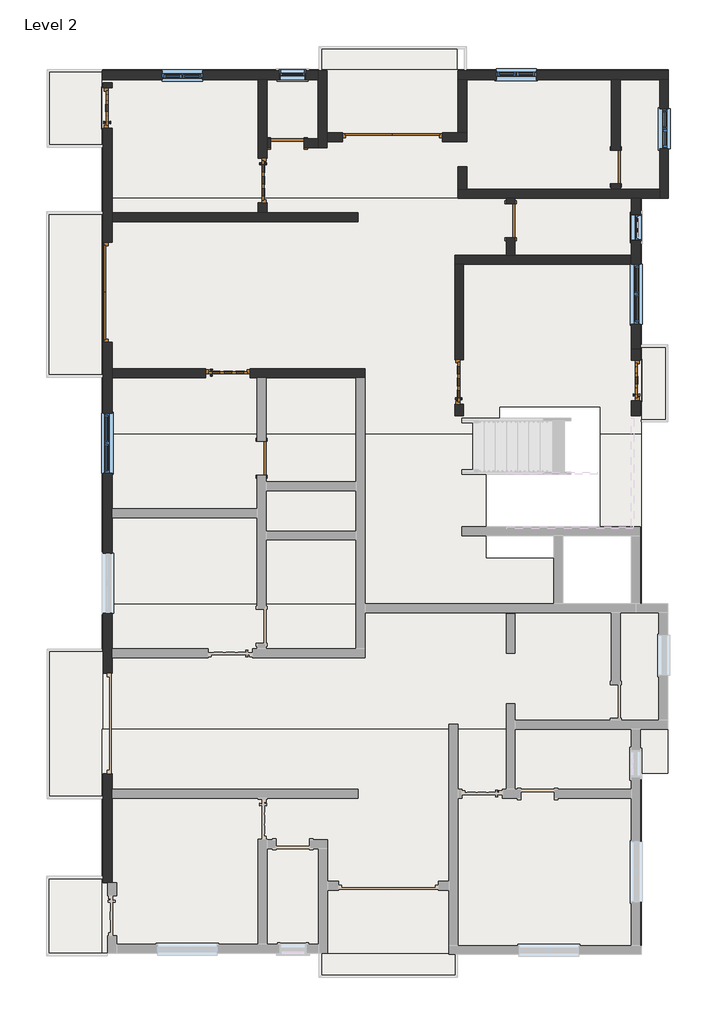
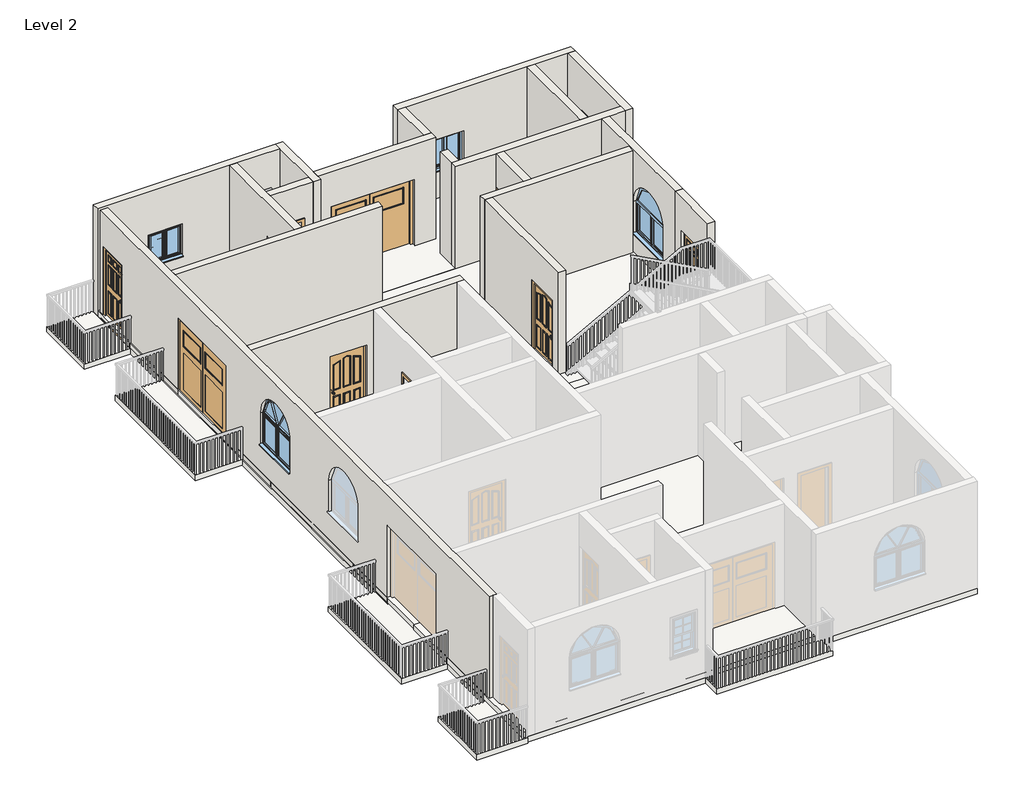
# One storey, part 2 of 7: 19 walls, 11 doors, 10 slabs, 7 windows, 5 roofs.
# Revit data of these elements (continued)
# Type "Windows_Dbl_w-Glazing_Bars : 910x910mm" (continued)
#   Type Mark = "33"
#   Operation = "DoublePanelVertical"
#   Construction Type Id = "GSP4R"
#   Manufacturer = "Revit"
#   Keynote = "L10"
#   Analytic Construction = "1/8 in Pilkington single glazing"
#   Wrap Layers (Ext) from Ext = 0' - 4.03543"
#   Wrap Layers (Int) from Ext = 0' - 6.98819"
#   Window Board Projection = 0' - 0.98425"
#   Window Board Extension = 0' - 0.98425"
#   Visual Light Transmittance = 0.9
#   Solar Heat Gain Coefficient = 0.78
#   Rough Width = 2' - 11.82677"
#   Rough Height = 2' - 11.82677"
#   Height = 2' - 11.82677"
#   Width = 2' - 11.82677"
#   Heat Transfer Coefficient (U) = 0.6496 BTU/(h·ft²·°F)
#   Glazing Thickness = 0' - 0.94488"
#   Glazing Bar Thickness = 0' - 0.7874"
#   FrameOffset - External = 0' - 1.9685"
#   Frame Depth = 0' - 2.55906"
#   Default Head Height = 6' - 10.67717"
#   Cill Depth = 0' - 3.44488"
#   Cavity Closer Width = 0' - 1.9685"
#   Cavity Closer Offset from Ext = 0' - 4.03543"
#   Cavity Closer Depth = 0' - 3.34646"
#   Vis - Glazing Bars = yes
#   Vis - Cavity Closers = yes
#   Define Thermal Properties by = 1
#   Material Trim = Window Frame
#   Material Glazing Bars = Window Frame
#   Material Glass = Glass
#   Material Frame = Window Frame
#   Wall Closure = (empty or 0)
# Elements 1, 2 (IfcDoor, "Doors_ExtSgl_5 : 910x2110mm")
#   Phase Created = New Construction
#   Materials on its faces: "Door - Panel", "Door - Handle", "Door - Frame/Mullion", "Door - Glazing"
# Elements 3, 4, 5 (IfcDoor, "Doors_ExtSgl_6 : 1010x2110mm")
#   Phase Created = New Construction
#   Materials on its faces: "Door - Panel", "Door - Handle", "Door - Frame/Mullion", "Door - Glazing"
# Element 6 (IfcDoor, "Doors_Garage_Timber_Side_Hung_Glazing : 2270x2050mm")
#   Phase Created = New Construction
#   Materials on its faces: "Door - Panel", "Door - Frame/Mullion", "Door - Glazing"
# Element 7 (IfcDoor, "Doors_Garage_Timber_Side_Hung_Glazing : 2270x2200mm")
#   Phase Created = New Construction
#   Materials on its faces: "Door - Panel", "Door - Frame/Mullion", "Door - Glazing"
# Elements 8, 9, 10, 11 (IfcDoor, "Single-Flush : 30\" x 80\"")
#   Phase Created = New Construction
#   Materials on its faces: "Door - Frame", "Door - Panel"
# Elements 12, 16 (IfcRoof, "Generic - 12\"")
#   built-in parameter 1001705 = 10.5 (stored number, unit not read)
#   built-in parameter 1001710 = 33615
#   Phase Created = New Construction
#   Materials on its faces: "Default Roof", "Earth"
# Element 13 (IfcRoof, "Generic - 12\"")
#   built-in parameter 1001705 = 10.5 (stored number, unit not read)
#   built-in parameter 1001710 = 33615
#   Phase Created = New Construction
#   Materials on its faces: "Default Roof"
# Element 14 (IfcRoof, "Generic - 12\"")
#   built-in parameter 1001705 = 10.5 (stored number, unit not read)
#   built-in parameter 1001710 = 33615
#   Phase Created = New Construction
#   Materials on its faces: "Default Roof", "Concrete, Lightweight"
# Element 15 (IfcRoof, "Generic - 12\"")
#   built-in parameter 1001705 = 10.5 (stored number, unit not read)
#   built-in parameter 1001710 = 33615
#   Phase Created = New Construction
#   Materials on its faces: "Default Roof", "Wood - Stained"
# Element 17 (IfcSlab, "Generic - 12\"")
#   Height Offset From Level = 0' - 0"
#   Phase Created = New Construction
#   Materials on its faces: "Default Floor", "Oak Flooring", "Concrete, Lightweight"
# Element 18 (IfcSlab, "Generic - 12\"")
#   Height Offset From Level = 0' - 0"
#   Phase Created = New Construction
#   Materials on its faces: "Default Floor", "Wood - Stained", "Concrete, Lightweight"
# Element 19 (IfcSlab, "Generic - 12\"")
#   Height Offset From Level = 0' - 0"
#   Phase Created = New Construction
#   Materials on its faces: "Default Floor", "Earth"
# Element 20 (IfcSlab, "Generic - 12\"")
#   Height Offset From Level = 0' - 0"
#   Phase Created = New Construction
#   Materials on its faces: "Default Floor", "mm"
# Elements 21, 22, 23, 24, 25 (IfcSlab, "Generic - 12\"")
#   Height Offset From Level = 0' - 0"
#   Phase Created = New Construction
#   Materials on its faces: "Default Floor"
# Element 26 (IfcSlab, "Generic - 12\"")
#   Height Offset From Level = 0' - 0"
#   Phase Created = New Construction
#   Materials on its faces: "Concrete, Lightweight", "Earth", "Default Floor"
# Elements 27, 31 (IfcWall, "Generic - 9\" w")
#   Top Offset = 0' - 0"
#   Base Offset = 0' - 0"
#   wall height = 10' - 0"
#   Phase Created = New Construction
#   Base Constraint = Level 2
#   Top Constraint = Level 3
#   Materials on its faces: "Default Wall", "Earth"
# Element 28 (IfcWall, "Generic - 9\" w")
#   Top Offset = 0' - 0"
#   Base Offset = 0' - 0"
#   wall height = 10' - 0"
#   Phase Created = New Construction
#   Base Constraint = Level 2
#   Top Constraint = Level 3
#   Materials on its faces: "Default Wall", "Wood - Stained"
# Element 29 (IfcWall, "Generic - 9\" w")
#   Top Offset = 0' - 0"
#   Base Offset = 0' - 0"
#   wall height = 10' - 0"
#   Phase Created = New Construction
#   Base Constraint = Level 2
#   Top Constraint = Level 3
#   Materials on its faces: "Default Wall", "Grass"
# Element 30 (IfcWall, "Generic - 9\" w")
#   Top Offset = 0' - 0"
#   Base Offset = 0' - 0"
#   wall height = 10' - 0"
#   Phase Created = New Construction
#   Base Constraint = Level 2
#   Top Constraint = Level 3
#   Materials on its faces: "Default Wall", "mm"
# Elements 32, 33, 35, 37, 38, 40, 41, 42, 43, 44, 45 (IfcWall, "Generic -4.5\" p")
#   Top Offset = 0' - 0"
#   Base Offset = 0' - 0"
#   wall height = 10' - 0"
#   Phase Created = New Construction
#   Base Constraint = Level 2
#   Top Constraint = Level 3
#   Materials on its faces: "Default Wall"
# Elements 34, 39 (IfcWall, "Generic -4.5\" p")
#   Top Offset = 0' - 0"
#   Base Offset = 0' - 0"
#   wall height = 10' - 0"
#   Phase Created = New Construction
#   Base Constraint = Level 2
#   Top Constraint = Level 3
#   Materials on its faces: "Default Wall", "Earth"
# Element 36 (IfcWall, "Generic -4.5\" p")
#   Top Offset = 0' - 0"
#   Base Offset = 0' - 0"
#   wall height = 10' - 0"
#   Phase Created = New Construction
#   Base Constraint = Level 2
#   Top Constraint = Level 3
#   Materials on its faces: "Default Wall", "Oak Flooring"
# Element 46 (IfcWindow, "Window-Double-Hung : 24\" x 42\"")
#   Mark = "24"
#   Window Inset = 0' - 0"
#   Interior Wall Closure = 0' - 1 1/2"
#   Frame Extension = 0' - 1 1/4"
#   Exterior Wall Closure = 0' - 0 1/2"
#   Interior Trim Visibility = yes
#   Indicator Visibility = yes
#   Exterior Trim Visibility = yes
#   Phase Created = New Construction
#   Materials on its faces: "Wood - Stained", "Glass", "Clad - White"
# Element 47 (IfcWindow, "Window-Double-Hung : 24\" x 42\"")
#   Mark = "30"
#   Window Inset = 0' - 0"
#   Interior Wall Closure = 0' - 1 1/2"
#   Frame Extension = 0' - 1 1/4"
#   Exterior Wall Closure = 0' - 0 1/2"
#   Interior Trim Visibility = yes
#   Indicator Visibility = yes
#   Exterior Trim Visibility = yes
#   Phase Created = New Construction
#   Materials on its faces: "Wood - Stained", "Glass", "Clad - White"
# Element 48 (IfcWindow, "Windows_Arched : 1360x910mm")
#   Mark = "20"
#   Phase Created = New Construction
#   Materials on its faces: "Window Frame", "Glass"
# Element 49 (IfcWindow, "Windows_Arched : 1360x910mm")
#   Mark = "31"
#   Phase Created = New Construction
#   Materials on its faces: "Window Frame", "Glass"
# Element 50 (IfcWindow, "Windows_Dbl_w-Glazing_Bars : 910x910mm")
#   Mark = "27"
#   Phase Created = New Construction
#   Materials on its faces: "Window Frame", "Glass"
# Element 51 (IfcWindow, "Windows_Dbl_w-Glazing_Bars : 910x910mm")
#   Mark = "28"
#   Phase Created = New Construction
#   Materials on its faces: "Window Frame", "Glass"
# Element 52 (IfcWindow, "Windows_Dbl_w-Glazing_Bars : 910x910mm")
#   Mark = "29"
#   Phase Created = New Construction
#   Materials on its faces: "Window Frame", "Glass"
# Materials
#   "Door - Glazing": colour RGB 0 0 255, transparency 0.75
#   "Door - Panel": class "Wood", colour RGB 210 159 95, transparency 0, Cost = 0
#   "Door - Frame/Mullion": class "Wood", colour RGB 212 179 113, transparency 0
#   "Door - Handle": colour RGB 0 0 0, transparency 0
#   "Door - Frame": colour RGB 118 70 51, transparency 0, Cost = 0
#   "Wood - Stained": class "Wood", colour RGB 224 178 126, transparency 0, Cost = 0
#   "Clad - White": class "Wood", colour RGB 242 242 238, transparency 0, Cost = 0
#   "Glass": class "Glass", colour RGB 0 128 192, transparency 0.75, Description = "Soda Lime Glass", Cost = 0
#   "Window Frame": colour RGB 249 249 249, transparency 0
#   "Default Roof": colour RGB 88 101 114, transparency 0, Cost = 0
#   "Earth": class "Generic", colour RGB 97 75 62, transparency 0, Description = "Soil", Cost = 0
#   "Concrete, Lightweight": class "Concrete", colour RGB 142 141 140, transparency 0, Description = "Lightweight concrete", Cost = 0
#   "Default Floor": colour RGB 128 128 128, transparency 0, Cost = 0
#   "Oak Flooring": class "Wood", colour RGB 216 169 114, transparency 0, Description = "Quercus Rubra", Cost = 0
#   "mm": class "Generic", colour RGB 128 64 0, transparency 0.5, Cost = 0
#   "Default Wall": colour RGB 128 128 128, transparency 0, Cost = 0
#   "Grass": class "Generic", colour RGB 104 137 66, transparency 0, Description = "Physical material.", Cost = 0
